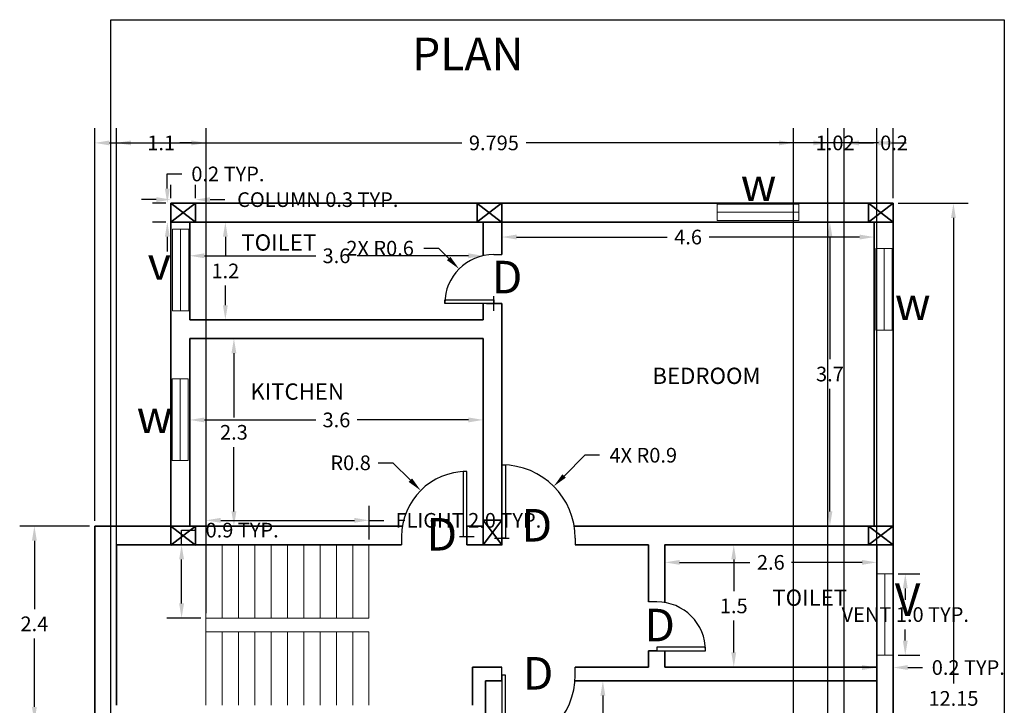
# Model space of a CAD drawing. Units: metres. Extents: x -16.7 to -4.6, y 24.4 to 40.
# Tile 2 of 2: x -16.7 to -4.6, y 31.6 to 40. Entities that reach past the tile are written whole.
import ezdxf

# ---------------------------------------------------------------- set-up
doc = ezdxf.new("R2010")
doc.units = ezdxf.units.M
doc.header["$MEASUREMENT"] = 0
for name, color, linetype, lineweight in [('A-ANNO-DIMS', 1, 'Continuous', 13), ('A-ANNO-TEXT', 5, 'Continuous', 18), ('A-ANNO-TTLB', 7, 'Continuous', 25), ('A-AREA-IDEN', 5, 'Continuous', 18), ('A-COLS', 7, 'Continuous', 35), ('A-WALL', 4, 'Continuous', 35), ('door', 3, 'Continuous', 25), ('stair', 2, 'Continuous', 18), ('window', 6, 'Continuous', 20)]:
    doc.layers.add(name, color=color, linetype=linetype, lineweight=lineweight)
doc.styles.get("Standard").update_dxf_attribs({"font": 'arial.ttf'})
doc.dimstyles.get("Standard").update_dxf_attribs({"dimtxt": 0.18, "dimasz": 0.18, "dimexe": 0.18, "dimexo": 0.0625, "dimgap": 0.09, "dimtad": 0, "dimtih": 1, "dimtoh": 1, "dimdec": 1, "dimzin": 0, "dimdsep": 46, "dimtxsty": 'Standard', "dimcen": 0.09, "dimadec": 0, "dimazin": 0, "dimtfac": 1, "dimtdec": 1, "dimtofl": 0, "dimtmove": 0, "dimatfit": 3, "dimfxl": 1, "dimtolj": 1, "dimtzin": 0, "dimarcsym": 0})

# ---------------------------------------------------------------- blocks, each defined once
blk = doc.blocks.new('*U2')
for p, q in [((-600, 0), (-600, -100)), ((0, 0), (0, -100))]:
    blk.add_line(p, q)
blk.add_lwpolyline([(0, 0), (0, 600), (-43.75, 600), (-43.75, 0)], close=True)
blk.add_arc((0, 0), 600, 90, 180)
blk = doc.blocks.new('*U3')
for p, q in [((0, 0), (0, 100)), ((900, 0), (900, 100))]:
    blk.add_line(p, q)
blk.add_lwpolyline([(0, 0), (0, -900), (43.75, -900), (43.75, 0)], close=True)
blk.add_arc((0, 0), 900, 270, 0)
blk = doc.blocks.new('*D5')
at = {"layer": 'A-ANNO-DIMS', "color": 0, "lineweight": -2, "transparency": 16777216}
for p, q in [((-14.1, 37.546), (-14.351, 37.546)), ((-14.171, 37.366), (-14.171, 37.127)), ((-14.171, 36.526), (-14.171, 36.766)), ((-14.1, 36.346), (-14.351, 36.346))]:
    blk.add_line(p, q, dxfattribs=at)
at = {"layer": 'A-ANNO-DIMS', "color": 0, "transparency": 16777216}
for points in [[(-14.201, 37.366), (-14.141, 37.366), (-14.171, 37.546)], [(-14.201, 36.526), (-14.141, 36.526), (-14.171, 36.346)]]:
    blk.add_solid(points, dxfattribs=at)
at = {"layer": 'Defpoints', "color": 0, "transparency": 16777216}
for p in [(-14.038, 37.546), (-14.171, 36.346), (-14.038, 36.346)]:
    blk.add_point(p, dxfattribs=at)
at = {"layer": 'A-ANNO-DIMS', "color": 0, "transparency": 16777216, "insert": (-14.171, 36.946), "char_height": 0.18, "attachment_point": 5}
blk.add_mtext('\\A1;1.2', dxfattribs=at)
blk = doc.blocks.new('*D6')
at = {"layer": 'A-ANNO-DIMS', "color": 0, "lineweight": -2, "transparency": 16777216}
for p, q in [((-14.608, 37.157), (-14.608, 37.312)), ((-11.008, 37.195), (-11.008, 37.312)), ((-14.428, 37.132), (-13.062, 37.132)), ((-11.188, 37.132), (-12.555, 37.132))]:
    blk.add_line(p, q, dxfattribs=at)
at = {"layer": 'A-ANNO-DIMS', "color": 0, "transparency": 16777216}
for points in [[(-14.428, 37.162), (-14.428, 37.102), (-14.608, 37.132)], [(-11.188, 37.162), (-11.188, 37.102), (-11.008, 37.132)]]:
    blk.add_solid(points, dxfattribs=at)
at = {"layer": 'Defpoints', "color": 0, "transparency": 16777216}
for p in [(-14.608, 37.095), (-11.008, 37.132), (-11.008, 37.132)]:
    blk.add_point(p, dxfattribs=at)
at = {"layer": 'A-ANNO-DIMS', "color": 0, "transparency": 16777216, "insert": (-12.808, 37.132), "char_height": 0.18, "attachment_point": 5}
blk.add_mtext('\\A1;3.6', dxfattribs=at)
blk = doc.blocks.new('*D7')
at = {"layer": 'A-ANNO-DIMS', "color": 0, "lineweight": -2, "transparency": 16777216}
for p, q in [((-10.778, 37.409), (-10.778, 37.542)), ((-6.208, 37.409), (-6.208, 37.542)), ((-10.598, 37.362), (-8.751, 37.362)), ((-6.388, 37.362), (-8.236, 37.362))]:
    blk.add_line(p, q, dxfattribs=at)
at = {"layer": 'A-ANNO-DIMS', "color": 0, "transparency": 16777216}
for points in [[(-10.598, 37.392), (-10.598, 37.332), (-10.778, 37.362)], [(-6.388, 37.392), (-6.388, 37.332), (-6.208, 37.362)]]:
    blk.add_solid(points, dxfattribs=at)
at = {"layer": 'Defpoints', "color": 0, "transparency": 16777216}
for p in [(-10.778, 37.346), (-6.208, 37.362), (-6.208, 37.346)]:
    blk.add_point(p, dxfattribs=at)
at = {"layer": 'A-ANNO-DIMS', "color": 0, "transparency": 16777216, "insert": (-8.493, 37.362), "char_height": 0.18, "attachment_point": 5}
blk.add_mtext('\\A1;4.6', dxfattribs=at)
blk = doc.blocks.new('*D8')
at = {"layer": 'A-ANNO-DIMS', "color": 0, "lineweight": -2, "transparency": 16777216}
for p, q in [((-6.815, 37.546), (-6.933, 37.546)), ((-6.753, 37.366), (-6.753, 35.863)), ((-6.753, 33.996), (-6.753, 35.499)), ((-6.815, 33.816), (-6.933, 33.816))]:
    blk.add_line(p, q, dxfattribs=at)
at = {"layer": 'A-ANNO-DIMS', "color": 0, "transparency": 16777216}
for points in [[(-6.783, 37.366), (-6.723, 37.366), (-6.753, 37.546)], [(-6.783, 33.996), (-6.723, 33.996), (-6.753, 33.816)]]:
    blk.add_solid(points, dxfattribs=at)
at = {"layer": 'Defpoints', "color": 0, "transparency": 16777216}
for p in [(-6.753, 37.546), (-6.753, 33.816), (-6.753, 33.816)]:
    blk.add_point(p, dxfattribs=at)
at = {"layer": 'A-ANNO-DIMS', "color": 0, "transparency": 16777216, "insert": (-6.753, 35.681), "char_height": 0.18, "attachment_point": 5}
blk.add_mtext('\\A1;3.7', dxfattribs=at)
blk = doc.blocks.new('*D9')
at = {"layer": 'A-ANNO-DIMS', "color": 0, "lineweight": -2, "transparency": 16777216}
for p, q in [((-7.995, 33.586), (-8.113, 33.586)), ((-7.933, 33.406), (-7.933, 33.018)), ((-7.933, 32.266), (-7.933, 32.655)), ((-7.995, 32.086), (-8.113, 32.086))]:
    blk.add_line(p, q, dxfattribs=at)
at = {"layer": 'A-ANNO-DIMS', "color": 0, "transparency": 16777216}
for points in [[(-7.963, 33.406), (-7.903, 33.406), (-7.933, 33.586)], [(-7.963, 32.266), (-7.903, 32.266), (-7.933, 32.086)]]:
    blk.add_solid(points, dxfattribs=at)
at = {"layer": 'Defpoints', "color": 0, "transparency": 16777216}
for p in [(-7.933, 33.586), (-7.933, 32.086), (-7.933, 32.086)]:
    blk.add_point(p, dxfattribs=at)
at = {"layer": 'A-ANNO-DIMS', "color": 0, "transparency": 16777216, "insert": (-7.933, 32.836), "char_height": 0.18, "attachment_point": 5}
blk.add_mtext('\\A1;1.5', dxfattribs=at)
blk = doc.blocks.new('*D10')
at = {"layer": 'A-ANNO-DIMS', "color": 0, "lineweight": -2, "transparency": 16777216}
for p, q in [((-8.778, 33.433), (-8.778, 33.55)), ((-6.178, 33.433), (-6.178, 33.55)), ((-8.598, 33.37), (-7.734, 33.37)), ((-6.358, 33.37), (-7.223, 33.37))]:
    blk.add_line(p, q, dxfattribs=at)
at = {"layer": 'A-ANNO-DIMS', "color": 0, "transparency": 16777216}
for points in [[(-8.598, 33.4), (-8.598, 33.34), (-8.778, 33.37)], [(-6.358, 33.4), (-6.358, 33.34), (-6.178, 33.37)]]:
    blk.add_solid(points, dxfattribs=at)
at = {"layer": 'Defpoints', "color": 0, "transparency": 16777216}
for p in [(-8.778, 33.37), (-8.778, 33.37), (-6.178, 33.37)]:
    blk.add_point(p, dxfattribs=at)
at = {"layer": 'A-ANNO-DIMS', "color": 0, "transparency": 16777216, "insert": (-7.478, 33.37), "char_height": 0.18, "attachment_point": 5}
blk.add_mtext('\\A1;2.6', dxfattribs=at)
blk = doc.blocks.new('*D12')
at = {"layer": 'A-ANNO-DIMS', "color": 0, "lineweight": -2, "transparency": 16777216}
for p, q in [((-9.041, 31.916), (-9.719, 31.916)), ((-9.539, 31.736), (-9.539, 30.098)), ((-9.539, 28.096), (-9.539, 29.735)), ((-9.041, 27.916), (-9.719, 27.916))]:
    blk.add_line(p, q, dxfattribs=at)
at = {"layer": 'A-ANNO-DIMS', "color": 0, "transparency": 16777216}
for points in [[(-9.569, 31.736), (-9.509, 31.736), (-9.539, 31.916)], [(-9.569, 28.096), (-9.509, 28.096), (-9.539, 27.916)]]:
    blk.add_solid(points, dxfattribs=at)
at = {"layer": 'Defpoints', "color": 0, "transparency": 16777216}
for p in [(-8.978, 31.916), (-9.539, 27.916), (-8.978, 27.916)]:
    blk.add_point(p, dxfattribs=at)
at = {"layer": 'A-ANNO-DIMS', "color": 0, "transparency": 16777216, "insert": (-9.539, 29.916), "char_height": 0.18, "attachment_point": 5}
blk.add_mtext('\\A1;4.0', dxfattribs=at)
blk = doc.blocks.new('*D17')
at = {"layer": 'A-ANNO-DIMS', "color": 0, "lineweight": -2, "transparency": 16777216}
for p, q in [((-14.608, 35.029), (-14.608, 35.298)), ((-11.008, 35.029), (-11.008, 35.298)), ((-14.428, 35.118), (-13.062, 35.118)), ((-11.188, 35.118), (-12.555, 35.118))]:
    blk.add_line(p, q, dxfattribs=at)
at = {"layer": 'A-ANNO-DIMS', "color": 0, "transparency": 16777216}
for points in [[(-14.428, 35.148), (-14.428, 35.088), (-14.608, 35.118)], [(-11.188, 35.148), (-11.188, 35.088), (-11.008, 35.118)]]:
    blk.add_solid(points, dxfattribs=at)
at = {"layer": 'Defpoints', "color": 0, "transparency": 16777216}
for p in [(-11.008, 35.118), (-14.608, 34.966), (-11.008, 34.966)]:
    blk.add_point(p, dxfattribs=at)
at = {"layer": 'A-ANNO-DIMS', "color": 0, "transparency": 16777216, "insert": (-12.808, 35.118), "char_height": 0.18, "attachment_point": 5}
blk.add_mtext('\\A1;3.6', dxfattribs=at)
blk = doc.blocks.new('*D18')
at = {"layer": 'A-ANNO-DIMS', "color": 0, "lineweight": -2, "transparency": 16777216}
for p, q in [((-14.168, 36.116), (-13.886, 36.116)), ((-14.066, 35.936), (-14.066, 35.148)), ((-14.066, 33.996), (-14.066, 34.784)), ((-14.168, 33.816), (-13.886, 33.816))]:
    blk.add_line(p, q, dxfattribs=at)
at = {"layer": 'A-ANNO-DIMS', "color": 0, "transparency": 16777216}
for points in [[(-14.096, 35.936), (-14.036, 35.936), (-14.066, 36.116)], [(-14.096, 33.996), (-14.036, 33.996), (-14.066, 33.816)]]:
    blk.add_solid(points, dxfattribs=at)
at = {"layer": 'Defpoints', "color": 0, "transparency": 16777216}
for p in [(-14.23, 36.116), (-14.23, 33.816), (-14.066, 33.816)]:
    blk.add_point(p, dxfattribs=at)
at = {"layer": 'A-ANNO-DIMS', "color": 0, "transparency": 16777216, "insert": (-14.066, 34.966), "char_height": 0.18, "attachment_point": 5}
blk.add_mtext('\\A1;2.3', dxfattribs=at)
blk = doc.blocks.new('WIN-1000')
blk.add_line((0, 0.1), (1, 0.1))
blk.add_lwpolyline([(0, 0), (1, 0), (1, 0.2), (0, 0.2)], close=True)
blk = doc.blocks.new('VENT-1000')
blk.add_line((0.1, 0), (0.1, 1))
blk.add_lwpolyline([(0.2, 0), (0.2, 1), (0, 1), (0, 0)], close=True)
blk = doc.blocks.new('COL-300x230')
for p, q in [((0, 0.23), (0.3, 0)), ((0, 0), (0.3, 0.23))]:
    blk.add_line(p, q)
blk.add_lwpolyline([(0, 0), (0, 0.23), (0.3, 0.23), (0.3, 0)], close=True)
blk = doc.blocks.new('STAIR-FLIGHT-2000x900')
for p, q in [((0.2, 0.9), (0.2, 0)), ((0.4, 0.9), (0.4, 0)), ((0.6, 0.9), (0.6, 0)), ((0.8, 0.9), (0.8, 0)), ((1, 0.9), (1, 0)), ((1.2, 0.9), (1.2, 0)), ((1.4, 0.9), (1.4, 0)), ((1.6, 0.9), (1.6, 0)), ((1.8, 0.9), (1.8, 0)), ((2, 0.9), (2, 0)), ((2, 0), (0, 0))]:
    blk.add_line(p, q)
blk = doc.blocks.new('*D25')
at = {"layer": 'A-ANNO-DIMS', "color": 0, "lineweight": -2, "transparency": 16777216}
for p, q in [((-5.916, 33.23), (-5.648, 33.23)), ((-5.828, 33.05), (-5.828, 32.912)), ((-5.828, 32.41), (-5.828, 32.548)), ((-5.916, 32.23), (-5.648, 32.23))]:
    blk.add_line(p, q, dxfattribs=at)
at = {"layer": 'A-ANNO-DIMS', "color": 0, "transparency": 16777216}
for points in [[(-5.858, 33.05), (-5.798, 33.05), (-5.828, 33.23)], [(-5.858, 32.41), (-5.798, 32.41), (-5.828, 32.23)]]:
    blk.add_solid(points, dxfattribs=at)
at = {"layer": 'Defpoints', "color": 0, "transparency": 16777216}
for p in [(-5.978, 33.23), (-5.828, 33.23), (-5.978, 32.23)]:
    blk.add_point(p, dxfattribs=at)
at = {"layer": 'A-ANNO-DIMS', "color": 0, "transparency": 16777216, "insert": (-5.828, 32.73), "char_height": 0.18, "attachment_point": 5}
blk.add_mtext('\\A1;VENT 1.0 TYP.', dxfattribs=at)
blk = doc.blocks.new('*D26')
at = {"layer": 'A-ANNO-DIMS', "color": 0, "lineweight": -2, "transparency": 16777216}
for p, q in [((-6.178, 32.168), (-6.178, 31.9)), ((-5.978, 32.168), (-5.978, 31.9)), ((-6.358, 32.08), (-6.538, 32.08)), ((-5.798, 32.08), (-5.618, 32.08))]:
    blk.add_line(p, q, dxfattribs=at)
at = {"layer": 'A-ANNO-DIMS', "color": 0, "transparency": 16777216}
for points in [[(-6.358, 32.11), (-6.358, 32.05), (-6.178, 32.08)], [(-5.798, 32.11), (-5.798, 32.05), (-5.978, 32.08)]]:
    blk.add_solid(points, dxfattribs=at)
at = {"layer": 'Defpoints', "color": 0, "transparency": 16777216}
for p in [(-6.178, 32.23), (-5.978, 32.23), (-5.978, 32.08)]:
    blk.add_point(p, dxfattribs=at)
at = {"layer": 'A-ANNO-DIMS', "color": 0, "transparency": 16777216, "insert": (-5.055, 32.08), "char_height": 0.18, "attachment_point": 5}
blk.add_mtext('\\A1;0.2 TYP.', dxfattribs=at)
blk = doc.blocks.new('*D27')
at = {"layer": 'A-ANNO-DIMS', "color": 0, "lineweight": -2, "transparency": 16777216}
for p, q in [((-14.838, 37.839), (-14.838, 38.001)), ((-14.538, 37.839), (-14.538, 38.001)), ((-15.018, 37.821), (-15.198, 37.821)), ((-14.358, 37.821), (-14.178, 37.821))]:
    blk.add_line(p, q, dxfattribs=at)
at = {"layer": 'A-ANNO-DIMS', "color": 0, "transparency": 16777216}
for points in [[(-15.018, 37.851), (-15.018, 37.791), (-14.838, 37.821)], [(-14.358, 37.851), (-14.358, 37.791), (-14.538, 37.821)]]:
    blk.add_solid(points, dxfattribs=at)
at = {"layer": 'Defpoints', "color": 0, "transparency": 16777216}
for p in [(-14.538, 37.821), (-14.838, 37.776), (-14.538, 37.776)]:
    blk.add_point(p, dxfattribs=at)
at = {"layer": 'A-ANNO-DIMS', "color": 0, "transparency": 16777216, "insert": (-13.037, 37.821), "char_height": 0.18, "attachment_point": 5}
blk.add_mtext('\\A1;COLUMN 0.3 TYP.', dxfattribs=at)
blk = doc.blocks.new('*D28')
at = {"layer": 'A-ANNO-DIMS', "color": 0, "lineweight": -2, "transparency": 16777216}
for p, q in [((-14.883, 37.956), (-14.883, 38.136)), ((-14.883, 38.136), (-14.703, 38.136)), ((-14.901, 37.776), (-15.063, 37.776)), ((-14.901, 37.546), (-15.063, 37.546)), ((-14.883, 37.366), (-14.883, 37.186))]:
    blk.add_line(p, q, dxfattribs=at)
at = {"layer": 'A-ANNO-DIMS', "color": 0, "transparency": 16777216}
for points in [[(-14.913, 37.956), (-14.853, 37.956), (-14.883, 37.776)], [(-14.913, 37.366), (-14.853, 37.366), (-14.883, 37.546)]]:
    blk.add_solid(points, dxfattribs=at)
at = {"layer": 'Defpoints', "color": 0, "transparency": 16777216}
for p in [(-14.883, 37.776), (-14.838, 37.776), (-14.838, 37.546)]:
    blk.add_point(p, dxfattribs=at)
at = {"layer": 'A-ANNO-DIMS', "color": 0, "transparency": 16777216, "insert": (-14.14, 38.136), "char_height": 0.18, "attachment_point": 5}
blk.add_mtext('\\A1;0.2 TYP.', dxfattribs=at)
blk = doc.blocks.new('*D29')
at = {"layer": 'A-ANNO-DIMS', "color": 0, "lineweight": -2, "transparency": 16777216}
for p, q in [((-14.408, 33.649), (-14.408, 34.066)), ((-12.408, 33.649), (-12.408, 34.066)), ((-14.228, 33.886), (-12.588, 33.886)), ((-12.408, 33.886), (-12.228, 33.886))]:
    blk.add_line(p, q, dxfattribs=at)
at = {"layer": 'A-ANNO-DIMS', "color": 0, "transparency": 16777216}
for points in [[(-14.228, 33.916), (-14.228, 33.856), (-14.408, 33.886)], [(-12.588, 33.916), (-12.588, 33.856), (-12.408, 33.886)]]:
    blk.add_solid(points, dxfattribs=at)
at = {"layer": 'Defpoints', "color": 0, "transparency": 16777216}
for p in [(-12.408, 33.886), (-14.408, 33.586), (-12.408, 33.586)]:
    blk.add_point(p, dxfattribs=at)
at = {"layer": 'A-ANNO-DIMS', "color": 0, "transparency": 16777216, "insert": (-11.189, 33.886), "char_height": 0.18, "attachment_point": 5}
blk.add_mtext('\\A1;FLIGHT 2.0 TYP.', dxfattribs=at)
blk = doc.blocks.new('*D30')
at = {"layer": 'A-ANNO-DIMS', "color": 0, "lineweight": -2, "transparency": 16777216}
for p, q in [((-14.708, 33.586), (-14.708, 33.766)), ((-14.708, 33.766), (-14.528, 33.766)), ((-14.471, 33.586), (-14.888, 33.586)), ((-14.708, 32.866), (-14.708, 33.406)), ((-14.471, 32.686), (-14.888, 32.686))]:
    blk.add_line(p, q, dxfattribs=at)
at = {"layer": 'A-ANNO-DIMS', "color": 0, "transparency": 16777216}
for points in [[(-14.738, 33.406), (-14.678, 33.406), (-14.708, 33.586)], [(-14.738, 32.866), (-14.678, 32.866), (-14.708, 32.686)]]:
    blk.add_solid(points, dxfattribs=at)
at = {"layer": 'Defpoints', "color": 0, "transparency": 16777216}
for p in [(-14.708, 33.586), (-14.408, 33.586), (-14.408, 32.686)]:
    blk.add_point(p, dxfattribs=at)
at = {"layer": 'A-ANNO-DIMS', "color": 0, "transparency": 16777216, "insert": (-13.965, 33.766), "char_height": 0.18, "attachment_point": 5}
blk.add_mtext('\\A1;0.9 TYP.', dxfattribs=at)
blk = doc.blocks.new('*D31')
at = {"layer": 'A-ANNO-DIMS', "color": 0, "lineweight": -2, "transparency": 16777216}
for p, q in [((-15.773, 33.879), (-15.773, 38.697)), ((-5.978, 37.839), (-5.978, 38.697)), ((-15.593, 38.517), (-11.27, 38.517)), ((-6.158, 38.517), (-10.482, 38.517))]:
    blk.add_line(p, q, dxfattribs=at)
at = {"layer": 'A-ANNO-DIMS', "color": 0, "transparency": 16777216}
for points in [[(-15.593, 38.547), (-15.593, 38.487), (-15.773, 38.517)], [(-6.158, 38.547), (-6.158, 38.487), (-5.978, 38.517)]]:
    blk.add_solid(points, dxfattribs=at)
at = {"layer": 'Defpoints', "color": 0, "transparency": 16777216}
for p in [(-5.978, 38.517), (-5.978, 37.776), (-15.773, 33.816)]:
    blk.add_point(p, dxfattribs=at)
at = {"layer": 'A-ANNO-DIMS', "color": 0, "transparency": 16777216, "insert": (-10.876, 38.517), "char_height": 0.18, "attachment_point": 5}
blk.add_mtext('\\A1;9.795', dxfattribs=at)
blk = doc.blocks.new('*D32')
at = {"layer": 'A-ANNO-DIMS', "color": 0, "lineweight": -2, "transparency": 16777216}
for p, q in [((-5.916, 37.776), (-5.057, 37.776)), ((-5.237, 37.596), (-5.237, 31.883)), ((-5.237, 25.806), (-5.237, 31.52)), ((-5.916, 25.626), (-5.057, 25.626))]:
    blk.add_line(p, q, dxfattribs=at)
at = {"layer": 'A-ANNO-DIMS', "color": 0, "transparency": 16777216}
for points in [[(-5.267, 37.596), (-5.207, 37.596), (-5.237, 37.776)], [(-5.267, 25.806), (-5.207, 25.806), (-5.237, 25.626)]]:
    blk.add_solid(points, dxfattribs=at)
at = {"layer": 'Defpoints', "color": 0, "transparency": 16777216}
for p in [(-5.978, 37.776), (-5.237, 37.776), (-5.978, 25.626)]:
    blk.add_point(p, dxfattribs=at)
at = {"layer": 'A-ANNO-DIMS', "color": 0, "transparency": 16777216, "insert": (-5.237, 31.701), "char_height": 0.18, "attachment_point": 5}
blk.add_mtext('\\A1;12.15', dxfattribs=at)
blk = doc.blocks.new('*D34')
at = {"layer": 'A-ANNO-DIMS', "color": 0, "lineweight": -2, "transparency": 16777216}
for p, q in [((-15.836, 33.816), (-16.694, 33.816)), ((-16.514, 33.636), (-16.514, 32.797)), ((-16.514, 31.596), (-16.514, 32.436)), ((-15.836, 31.416), (-16.694, 31.416))]:
    blk.add_line(p, q, dxfattribs=at)
at = {"layer": 'A-ANNO-DIMS', "color": 0, "transparency": 16777216}
for points in [[(-16.544, 33.636), (-16.484, 33.636), (-16.514, 33.816)], [(-16.544, 31.596), (-16.484, 31.596), (-16.514, 31.416)]]:
    blk.add_solid(points, dxfattribs=at)
at = {"layer": 'Defpoints', "color": 0, "transparency": 16777216}
for p in [(-16.514, 33.816), (-15.773, 33.816), (-15.773, 31.416)]:
    blk.add_point(p, dxfattribs=at)
at = {"layer": 'A-ANNO-DIMS', "color": 0, "transparency": 16777216, "insert": (-16.514, 32.616), "char_height": 0.18, "attachment_point": 5}
blk.add_mtext('\\A1;2.4', dxfattribs=at)
blk = doc.blocks.new('*D35')
at = {"layer": 'A-ANNO-DIMS', "color": 0, "lineweight": -2, "transparency": 16777216}
for p, q in [((-15.508, 31.679), (-15.508, 38.697)), ((-14.408, 32.749), (-14.408, 38.697)), ((-15.328, 38.517), (-15.187, 38.517)), ((-14.588, 38.517), (-14.73, 38.517))]:
    blk.add_line(p, q, dxfattribs=at)
at = {"layer": 'A-ANNO-DIMS', "color": 0, "transparency": 16777216}
for points in [[(-15.328, 38.547), (-15.328, 38.487), (-15.508, 38.517)], [(-14.588, 38.547), (-14.588, 38.487), (-14.408, 38.517)]]:
    blk.add_solid(points, dxfattribs=at)
at = {"layer": 'Defpoints', "color": 0, "transparency": 16777216}
for p in [(-14.408, 38.517), (-14.408, 32.686), (-15.508, 31.616)]:
    blk.add_point(p, dxfattribs=at)
at = {"layer": 'A-ANNO-DIMS', "color": 0, "transparency": 16777216, "insert": (-14.958, 38.517), "char_height": 0.18, "attachment_point": 5}
blk.add_mtext('\\A1;1.1', dxfattribs=at)
blk = doc.blocks.new('*D38')
at = {"layer": 'A-ANNO-DIMS', "color": 0, "lineweight": -2, "transparency": 16777216}
for p, q in [((-6.778, 27.789), (-6.778, 38.697)), ((-6.578, 27.789), (-6.578, 38.697)), ((-6.958, 38.517), (-7.138, 38.517)), ((-6.398, 38.517), (-6.218, 38.517))]:
    blk.add_line(p, q, dxfattribs=at)
at = {"layer": 'A-ANNO-DIMS', "color": 0, "transparency": 16777216}
for points in [[(-6.958, 38.547), (-6.958, 38.487), (-6.778, 38.517)], [(-6.398, 38.547), (-6.398, 38.487), (-6.578, 38.517)]]:
    blk.add_solid(points, dxfattribs=at)
at = {"layer": 'Defpoints', "color": 0, "transparency": 16777216}
for p in [(-6.578, 38.517), (-6.778, 27.726), (-6.578, 27.726)]:
    blk.add_point(p, dxfattribs=at)
at = {"layer": 'A-ANNO-DIMS', "color": 0, "transparency": 16777216, "insert": (-5.966, 38.517), "char_height": 0.18, "attachment_point": 5}
blk.add_mtext('\\A1;0.2', dxfattribs=at)
blk = doc.blocks.new('*D39')
at = {"layer": 'A-ANNO-DIMS', "color": 0, "lineweight": -2, "transparency": 16777216}
for p, q in [((-7.199, 27.984), (-7.199, 38.697)), ((-6.178, 27.979), (-6.178, 38.697)), ((-7.379, 38.517), (-7.559, 38.517)), ((-5.998, 38.517), (-5.818, 38.517))]:
    blk.add_line(p, q, dxfattribs=at)
at = {"layer": 'A-ANNO-DIMS', "color": 0, "transparency": 16777216}
for points in [[(-7.379, 38.547), (-7.379, 38.487), (-7.199, 38.517)], [(-5.998, 38.547), (-5.998, 38.487), (-6.178, 38.517)]]:
    blk.add_solid(points, dxfattribs=at)
at = {"layer": 'Defpoints', "color": 0, "transparency": 16777216}
for p in [(-7.199, 38.517), (-7.199, 27.921), (-6.178, 27.916)]:
    blk.add_point(p, dxfattribs=at)
at = {"layer": 'A-ANNO-DIMS', "color": 0, "transparency": 16777216, "insert": (-6.689, 38.517), "char_height": 0.18, "attachment_point": 5}
blk.add_mtext('\\A1;1.02', dxfattribs=at)
blk = doc.blocks.new('*D41')
at = {"layer": 'A-ANNO-DIMS', "color": 0, "lineweight": -2, "transparency": 16777216}
for p, q in [((-9.76, 34.685), (-10.015, 34.43)), ((-9.58, 34.685), (-9.76, 34.685)), ((-10.778, 33.576), (-10.778, 33.756)), ((-10.868, 33.666), (-10.688, 33.666))]:
    blk.add_line(p, q, dxfattribs=at)
at = {"layer": 'A-ANNO-DIMS', "color": 0, "transparency": 16777216}
blk.add_solid([(-10.036, 34.451), (-9.994, 34.409), (-10.142, 34.303)], dxfattribs=at)
at = {"layer": 'Defpoints', "color": 0, "transparency": 16777216}
for p in [(-10.142, 34.303), (-10.778, 33.666)]:
    blk.add_point(p, dxfattribs=at)
at = {"layer": 'A-ANNO-DIMS', "color": 0, "transparency": 16777216, "insert": (-9.043, 34.685), "char_height": 0.18, "attachment_point": 5}
blk.add_mtext('\\A1;4X R0.9', dxfattribs=at)
blk = doc.blocks.new('*D42')
at = {"layer": 'A-ANNO-DIMS', "color": 0, "lineweight": -2, "transparency": 16777216}
for p, q in [((-12.294, 34.592), (-12.114, 34.592)), ((-12.114, 34.592), (-11.901, 34.379)), ((-11.208, 33.596), (-11.208, 33.776)), ((-11.298, 33.686), (-11.118, 33.686))]:
    blk.add_line(p, q, dxfattribs=at)
at = {"layer": 'A-ANNO-DIMS', "color": 0, "transparency": 16777216}
blk.add_solid([(-11.88, 34.401), (-11.923, 34.358), (-11.774, 34.252)], dxfattribs=at)
at = {"layer": 'Defpoints', "color": 0, "transparency": 16777216}
for p in [(-11.774, 34.252), (-11.208, 33.686)]:
    blk.add_point(p, dxfattribs=at)
at = {"layer": 'A-ANNO-DIMS', "color": 0, "transparency": 16777216, "insert": (-12.634, 34.592), "char_height": 0.18, "attachment_point": 5}
blk.add_mtext('\\A1;R0.8', dxfattribs=at)
blk = doc.blocks.new('*D43')
at = {"layer": 'A-ANNO-DIMS', "color": 0, "lineweight": -2, "transparency": 16777216}
for p, q in [((-11.737, 37.225), (-11.557, 37.225)), ((-11.557, 37.225), (-11.43, 37.098)), ((-10.878, 36.456), (-10.878, 36.636)), ((-10.968, 36.546), (-10.788, 36.546))]:
    blk.add_line(p, q, dxfattribs=at)
at = {"layer": 'A-ANNO-DIMS', "color": 0, "transparency": 16777216}
blk.add_solid([(-11.409, 37.119), (-11.451, 37.077), (-11.303, 36.971)], dxfattribs=at)
at = {"layer": 'Defpoints', "color": 0, "transparency": 16777216}
for p in [(-11.303, 36.971), (-10.878, 36.546)]:
    blk.add_point(p, dxfattribs=at)
at = {"layer": 'A-ANNO-DIMS', "color": 0, "transparency": 16777216, "insert": (-12.272, 37.225), "char_height": 0.18, "attachment_point": 5}
blk.add_mtext('\\A1;2X R0.6', dxfattribs=at)

msp = doc.modelspace()

# ---------------------------------------------------------------- linework, layer by layer
at = {"layer": 'A-ANNO-TTLB'}
msp.add_lwpolyline([(-15.5749, 40.0289), (-4.6131, 40.0289), (-4.6131, 24.4246), (-15.5749, 24.4246)], close=True, dxfattribs=at)
at = {"layer": 'A-COLS'}
for p, q in [((-11.0844, 37.7764), (-10.7844, 37.5464)), ((-11.0844, 37.5464), (-10.7844, 37.7764)), ((-6.2787, 37.7764), (-5.9787, 37.5464)), ((-6.2787, 37.5464), (-5.9787, 37.7764)), ((-14.8385, 33.8127), (-14.5385, 33.5827)), ((-14.8385, 33.5827), (-14.5385, 33.8127))]:
    msp.add_line(p, q, dxfattribs=at)
for points in [[(-11.0794, 37.5464), (-11.0794, 37.7764), (-10.7794, 37.7764), (-10.7794, 37.5464)], [(-6.2783, 37.5464), (-6.2783, 37.7764), (-5.9783, 37.7764), (-5.9783, 37.5464)], [(-14.8385, 33.5854), (-14.8385, 33.8154), (-14.5385, 33.8154), (-14.5385, 33.5854)]]:
    msp.add_lwpolyline(points, close=True, dxfattribs=at)
at = {"layer": 'A-WALL'}
for p, q in [((-14.8385, 36.1164), (-14.8385, 37.7764)), ((-14.8385, 37.7764), (-10.7785, 37.7764)), ((-11.2385, 37.7764), (-5.9785, 37.7764)), ((-5.9785, 37.7764), (-5.9785, 33.5864)), ((-14.6085, 36.3464), (-14.6085, 37.5464)), ((-14.6085, 37.5464), (-11.0085, 37.5464)), ((-11.0085, 37.5464), (-11.0085, 37.1322)), ((-11.0085, 37.1322), (-11.0085, 37.5464)), ((-10.7785, 37.5464), (-10.7785, 37.1464)), ((-10.7785, 37.5464), (-6.2085, 37.5464)), ((-10.7785, 37.1464), (-10.7785, 37.5464)), ((-6.2085, 37.5464), (-6.2085, 33.8164)), ((-11.0085, 36.5464), (-11.0085, 36.3464)), ((-11.0085, 36.3464), (-11.0085, 36.5464)), ((-10.7785, 33.5864), (-10.7785, 36.5464)), ((-10.7785, 36.1164), (-10.7785, 36.5464)), ((-14.8385, 33.8164), (-14.8385, 36.3464)), ((-11.0085, 36.3464), (-14.6085, 36.3464)), ((-11.0085, 36.1164), (-14.6085, 36.1164)), ((-14.6085, 33.8164), (-14.6085, 36.1164)), ((-14.6085, 36.1164), (-11.0085, 36.1164)), ((-11.0085, 36.1164), (-11.0085, 33.8164)), ((-14.8385, 33.8164), (-15.7735, 33.8164)), ((-15.7735, 31.4164), (-15.7735, 33.8164)), ((-11.9979, 33.8164), (-14.6085, 33.8164)), ((-11.2085, 33.8164), (-11.2085, 33.5864)), ((-11.0085, 33.8164), (-11.2085, 33.8164)), ((-6.2085, 33.8164), (-9.8911, 33.8164)), ((-14.6085, 33.5864), (-15.5085, 33.5864)), ((-15.5085, 33.5864), (-15.5085, 31.6164)), ((-12.0085, 33.5864), (-14.8385, 33.5864)), ((-11.2085, 33.5864), (-10.7785, 33.5864)), ((-9.8785, 33.5864), (-8.9785, 33.5864)), ((-8.7785, 33.5864), (-6.1785, 33.5864)), ((-11.1385, 32.0864), (-10.7785, 32.0864)), ((-11.1385, 31.6164), (-11.1385, 32.0864)), ((-9.8785, 32.0864), (-8.9785, 32.0864)), ((-5.9785, 32.0864), (-5.9785, 25.6264))]:
    msp.add_line(p, q, dxfattribs=at)
for points in [[(-5.9785, 33.8164), (-5.9785, 31.9164)], [(-8.9785, 32.8864), (-8.9785, 33.5864)], [(-8.7785, 32.8781), (-8.7785, 33.5864), (-6.1785, 33.5864), (-6.1785, 32.0864), (-8.7785, 32.0864), (-8.7785, 32.2864)], [(-8.9785, 32.0864), (-8.9785, 32.2864)], [(-10.7785, 27.9164), (-10.9785, 27.9164), (-10.9785, 31.9164), (-10.7785, 31.9164)], [(-9.8812, 31.9164), (-6.1785, 31.9164), (-6.1785, 27.9164), (-9.883, 27.9164)], [(-6.1785, 31.9164), (-8.9785, 31.9164)]]:
    msp.add_lwpolyline(points, dxfattribs=at)
at = {"layer": 'door'}
for p, q in [((-10.8785, 37.1464), (-10.7785, 37.1464)), ((-10.7785, 36.5464), (-11.0085, 36.5464)), ((-10.8785, 36.5464), (-10.7785, 36.5464)), ((-10.7785, 33.8164), (-10.7785, 33.5864)), ((-12.0085, 33.6864), (-12.0085, 33.5864)), ((-11.2085, 33.6864), (-11.2085, 33.5864)), ((-10.7785, 33.6664), (-10.7785, 33.5864)), ((-9.8785, 33.6664), (-9.8785, 33.5864)), ((-8.9785, 32.2864), (-8.7785, 32.2864)), ((-10.7785, 31.9164), (-10.7785, 32.0864))]:
    msp.add_line(p, q, dxfattribs=at)
for points in [[(-10.8785, 36.5464), (-11.4785, 36.5464), (-11.4785, 36.5902), (-10.8785, 36.5902)], [(-10.7785, 33.6664), (-10.7785, 34.5664), (-10.7347, 34.5664), (-10.7347, 33.6664)], [(-11.2085, 33.6864), (-11.2085, 34.4864), (-11.2522, 34.4864), (-11.2522, 33.6864)]]:
    msp.add_lwpolyline(points, close=True, dxfattribs=at)
for centre, radius, start, end in [((-10.8785, 36.5464), 0.6, 90, 180), ((-10.7785, 33.6664), 0.9, 0, 90), ((-11.2085, 33.6864), 0.8, 90, 180)]:
    msp.add_arc(centre, radius, start, end, dxfattribs=at)
at = {"layer": 'stair'}
msp.add_line((-14.4085, 33.5864), (-14.4085, 31.6164), dxfattribs=at)

# ---------------------------------------------------------------- block references
at = {"layer": 'A-COLS'}
for p in [(-14.8385, 37.5464), (-6.2785, 33.5864)]:
    msp.add_blockref('COL-300x230', p, dxfattribs=at)
at = {"layer": 'A-COLS', "rotation": 269.9999999999972}
msp.add_blockref('COL-300x230', (-11.0085, 33.8864), dxfattribs=at)
at = {"layer": 'door', "xscale": 0.001, "yscale": 0.001, "zscale": 0.001, "rotation": 270}
msp.add_blockref('*U2', (-8.8785, 32.2864), dxfattribs=at)
at = {"layer": 'door', "xscale": 0.001, "yscale": 0.001, "zscale": 0.001}
msp.add_blockref('*U3', (-10.7785, 31.9864), dxfattribs=at)
at = {"layer": 'stair'}
msp.add_blockref('STAIR-FLIGHT-2000x900', (-14.4085, 32.6864), dxfattribs=at)
at = {"layer": 'stair', "extrusion": (0, 0, -1), "zscale": -1, "rotation": 180}
msp.add_blockref('STAIR-FLIGHT-2000x900', (14.4085, 32.5164), dxfattribs=at)
at = {"layer": 'window'}
for name, p in [('WIN-1000', (-8.1358, 37.5659)), ('VENT-1000', (-14.82, 36.4567)), ('VENT-1000', (-6.178, 32.2303))]:
    msp.add_blockref(name, p, dxfattribs=at)
for p, rotation in [((-5.9892, 36.2209), 89.99999999999945), ((-14.6256, 34.6203), 89.99999999999902)]:
    msp.add_blockref('WIN-1000', p, dxfattribs=dict(at, rotation=rotation))

# ---------------------------------------------------------------- texts
at = {"layer": 'A-ANNO-TEXT', "char_height": 0.4, "attachment_point": 1}
for s, width, insert in [('PLAN', 5.518236, (-11.8792, 39.8088)), ('w', 0.312835, (-7.8475, 38.2063)), ('v', 0.312835, (-15.1238, 37.2398)), ('D', 0.312835, (-10.9024, 37.0705)), ('w', 0.312835, (-5.956, 36.7457)), ('w', 0.312835, (-15.2588, 35.3584)), ('D', 0.312835, (-10.537, 34.0254)), ('D', 0.312835, (-11.7025, 33.915)), ('V', 0.312835, (-5.957, 33.1132)), ('D', 0.312835, (-9.0299, 32.8011)), ('D', 0.312835, (-10.5219, 32.209))]:
    msp.add_mtext_dynamic_manual_height_columns(s, width=width, gutter_width=1, heights=[0], dxfattribs=dict(at, insert=insert))
at = {"layer": 'A-AREA-IDEN', "char_height": 0.2, "attachment_point": 1}
for s, width, insert in [('TOILET', 0.943028, (-13.9745, 37.3952)), ('BEDROOM', 0.273342, (-8.9313, 35.7591)), ('KITCHEN', 0.273342, (-13.8651, 35.566)), ('TOILET', 0.273342, (-7.4601, 33.037))]:
    msp.add_mtext_dynamic_manual_height_columns(s, width=width, gutter_width=1, heights=[0], dxfattribs=dict(at, insert=insert))

# ---------------------------------------------------------------- dimensions: what is measured, and where the dimension line sits
at = {"layer": 'A-ANNO-DIMS'}
for base, p1, p2, override, picture, middle in [((-5.9783, 38.5174), (-15.7735, 33.8164), (-5.9783, 37.7764), {"dimdec": 3, "dimlfac": 1, "dimrnd": 0, "dimzin": 0, "dimdsep": 46, "dimlunit": 2}, '*D31', (-10.8759, 38.5174)), ((-14.4085, 38.5174), (-15.5085, 31.6164), (-14.4085, 32.6864), {"dimdec": 1, "dimlfac": 1, "dimrnd": 0, "dimzin": 0, "dimdsep": 46, "dimlunit": 2}, '*D35', (-14.9585, 38.5174)), ((-7.1986, 38.5174), (-6.1785, 27.9164), (-7.1986, 27.9212), {"dimdec": 2, "dimlfac": 1, "dimrnd": 0, "dimzin": 0, "dimdsep": 46, "dimlunit": 2}, '*D39', (-6.6885, 38.5174)), ((-6.5785, 38.5174), (-6.7785, 27.7264), (-6.5785, 27.7264), {"dimdec": 1, "dimlfac": 1, "dimrnd": 0, "dimzin": 0, "dimdsep": 46, "dimlunit": 2}, '*D38', (-5.9656, 38.5174)), ((-6.2085, 37.3615), (-10.7785, 37.3464), (-6.2085, 37.3464), {"dimclrd": 0, "dimclre": 0, "dimclrt": 0}, '*D7', (-8.4935, 37.3615)), ((-11.0085, 37.1322), (-14.6085, 37.0945), (-11.0085, 37.1322), {"dimclrd": 0, "dimclre": 0, "dimclrt": 0}, '*D6', (-12.8085, 37.1322)), ((-11.0085, 35.118), (-14.6085, 34.9664), (-11.0085, 34.9664), {"dimclrd": 0, "dimclre": 0, "dimclrt": 0}, '*D17', (-12.8085, 35.118)), ((-8.7785, 33.3702), (-6.1785, 33.3702), (-8.7785, 33.3702), {"dimclrd": 0, "dimclre": 0, "dimclrt": 0}, '*D10', (-7.4785, 33.3702))]:
    dim = msp.add_linear_dim(base=base, p1=p1, p2=p2, dimstyle='Standard', override=override, dxfattribs=at)
    dim.commit()
    dim.dimension.update_dxf_attribs({"geometry": picture, "text_midpoint": middle})
for base, p1, p2, text, picture, middle in [((-14.8835, 37.7764), (-14.8385, 37.5464), (-14.8385, 37.7764), '<> TYP.', '*D28', (-14.1405, 38.1364)), ((-14.7085, 33.5864), (-14.4085, 32.6864), (-14.4085, 33.5864), '<> TYP.', '*D30', (-13.9655, 33.7664)), ((-5.828, 33.2303), (-5.978, 32.2303), (-5.978, 33.2303), 'VENT <> TYP.', '*D25', (-5.828, 32.7303))]:
    dim = msp.add_linear_dim(base=base, p1=p1, p2=p2, angle=90, text=text, dimstyle='Standard', override={"dimdec": 1, "dimlfac": 1, "dimrnd": 0, "dimzin": 0, "dimdsep": 46, "dimlunit": 2}, dxfattribs=at)
    dim.commit()
    dim.dimension.update_dxf_attribs({"geometry": picture, "text_midpoint": middle})
for base, p1, p2, text, picture, middle in [((-14.5385, 37.8214), (-14.8385, 37.7764), (-14.5385, 37.7764), 'COLUMN <> TYP.', '*D27', (-13.0367, 37.8214)), ((-12.4085, 33.8864), (-14.4085, 33.5864), (-12.4085, 33.5864), 'FLIGHT <> TYP.', '*D29', (-11.1886, 33.8864)), ((-5.978, 32.0803), (-6.178, 32.2303), (-5.978, 32.2303), '<> TYP.', '*D26', (-5.055, 32.0803))]:
    dim = msp.add_linear_dim(base=base, p1=p1, p2=p2, text=text, dimstyle='Standard', override={"dimdec": 1, "dimlfac": 1, "dimrnd": 0, "dimzin": 0, "dimdsep": 46, "dimlunit": 2}, dxfattribs=at)
    dim.commit()
    dim.dimension.update_dxf_attribs({"geometry": picture, "text_midpoint": middle})
for base, p1, p2, override, picture, middle in [((-5.237, 37.7764), (-5.9785, 25.6264), (-5.9783, 37.7764), {"dimdec": 2, "dimlfac": 1, "dimrnd": 0, "dimzin": 0, "dimdsep": 46, "dimlunit": 2}, '*D32', (-5.237, 31.7014)), ((-14.1711, 36.3464), (-14.0378, 37.5464), (-14.0378, 36.3464), {"dimclrd": 0, "dimclre": 0, "dimclrt": 0}, '*D5', (-14.1711, 36.9464)), ((-6.7526, 33.8164), (-6.7526, 37.5464), (-6.7526, 33.8164), {"dimclrd": 0, "dimclre": 0, "dimclrt": 0}, '*D8', (-6.7526, 35.6814)), ((-14.066, 33.8164), (-14.2305, 36.1164), (-14.2305, 33.8164), {"dimclrd": 0, "dimclre": 0, "dimclrt": 0}, '*D18', (-14.066, 34.9664)), ((-16.5145, 33.8164), (-15.7735, 31.4164), (-15.7735, 33.8164), {"dimdec": 1, "dimlfac": 1, "dimrnd": 0, "dimzin": 0, "dimdsep": 46, "dimlunit": 2}, '*D34', (-16.5145, 32.6164)), ((-7.9327, 32.0864), (-7.9327, 33.5864), (-7.9327, 32.0864), {"dimclrd": 0, "dimclre": 0, "dimclrt": 0}, '*D9', (-7.9327, 32.8364)), ((-9.5386, 27.9164), (-8.9785, 31.9164), (-8.9785, 27.9164), {"dimclrd": 0, "dimclre": 0, "dimclrt": 0}, '*D12', (-9.5386, 29.9164))]:
    dim = msp.add_linear_dim(base=base, p1=p1, p2=p2, angle=90, dimstyle='Standard', override=override, dxfattribs=at)
    dim.commit()
    dim.dimension.update_dxf_attribs({"geometry": picture, "text_midpoint": middle})
dim = msp.add_radius_dim(center=(-10.8785, 36.5464), mpoint=(-11.3027, 36.9707), text='2X <>', dimstyle='Standard', override={"dimdec": 1, "dimlfac": 1, "dimrnd": 0, "dimzin": 0, "dimdsep": 46, "dimlunit": 2}, dxfattribs=at)
dim.commit()
dim.dimension.update_dxf_attribs({"geometry": '*D43', "text_midpoint": (-12.2721, 37.2253)})
dim = msp.add_radius_dim(center=(-10.7785, 33.6664), mpoint=(-10.1421, 34.3029), text='4X <>', dimstyle='Standard', override={"dimdec": 1, "dimlfac": 1, "dimrnd": 0, "dimzin": 0, "dimdsep": 46, "dimlunit": 2}, dxfattribs=at)
dim.commit()
dim.dimension.update_dxf_attribs({"geometry": '*D41', "text_midpoint": (-9.0431, 34.6847), "dimtype": 164})
dim = msp.add_radius_dim(center=(-11.2085, 33.6864), mpoint=(-11.7742, 34.2522), dimstyle='Standard', override={"dimdec": 1, "dimlfac": 1, "dimrnd": 0, "dimzin": 0, "dimdsep": 46, "dimlunit": 2}, dxfattribs=at)
dim.commit()
dim.dimension.update_dxf_attribs({"geometry": '*D42', "text_midpoint": (-12.6337, 34.5916), "dimtype": 164})

doc.saveas('drawing.dxf')
